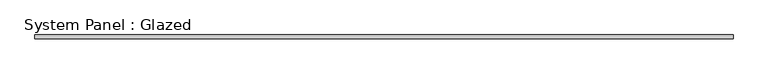
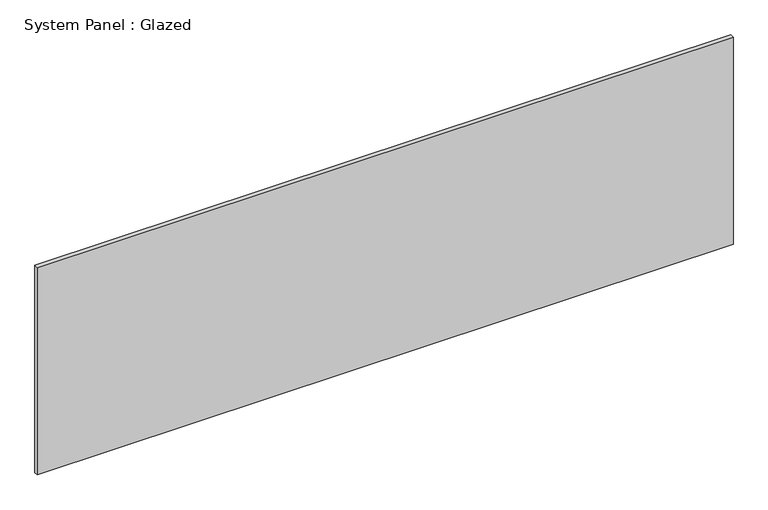
"""IFC4 building model written with IfcOpenShell, lengths in millimetres: plate geometry, System Panel : Glazed."""

from ifc_helpers import new_model, si_unit, origin, origin_with_axes, place, context, project, spatial, polyline, outline, extrude, source, transform, mapped, element, save


def system_panel_glazed_4eae45b3(model_context):
    return source(origin(), model_context, "Body", "SweptSolid", [
        extrude(outline(polyline([(2421.1302398, 19.05), (-2421.1302398, 19.05), (-2421.1302398, 44.45), (2421.1302398, 44.45), (2421.1302398, 19.05)])), origin_with_axes(), (0.0, 0.0, 1.0), 1524.0),
    ])


if __name__ == "__main__":
    model = new_model("IFC4")
    model_context = context("Model", 3, world=origin())
    ifc_project = project(units=[si_unit("LENGTHUNIT", "METRE", prefix="MILLI")], contexts=[model_context])
    site = spatial("IfcSite", under=ifc_project)
    building = spatial("IfcBuilding", under=site)
    placement = place(None, origin())
    system_panel_glazed_shape = system_panel_glazed_4eae45b3(model_context)
    element("IfcPlate", 1, ObjectType="System Panel : Glazed", at=placement, inside=building, context=model_context, shape_type="MappedRepresentation", body=[
        mapped(system_panel_glazed_shape, transform((0.0, 0.0, 0.0), x_axis=(1.0, 0.0, 0.0), y_axis=(0.0, 1.0, 0.0), z_axis=(0.0, 0.0, 1.0))),
    ])
    save(model, "model.ifc")

# Revit data of these elements
# Type "System Panel : Glazed"
#   Construction Type Id = "GSP4R"
#   Analytic Construction = "1/8 in Pilkington single glazing"
#   Visual Light Transmittance = 0.9
#   Solar Heat Gain Coefficient = 0.86
#   Heat Transfer Coefficient (U) = 1.18115 BTU/(h·ft²·°F)
# Element 1 (IfcPlate, "System Panel : Glazed")
#   Materials on its faces: "Glass"
# Materials
#   "Glass": class "Glass", colour RGB 0 128 192, transparency 0.75, Description = "Soda Lime Glass", Cost = 0
